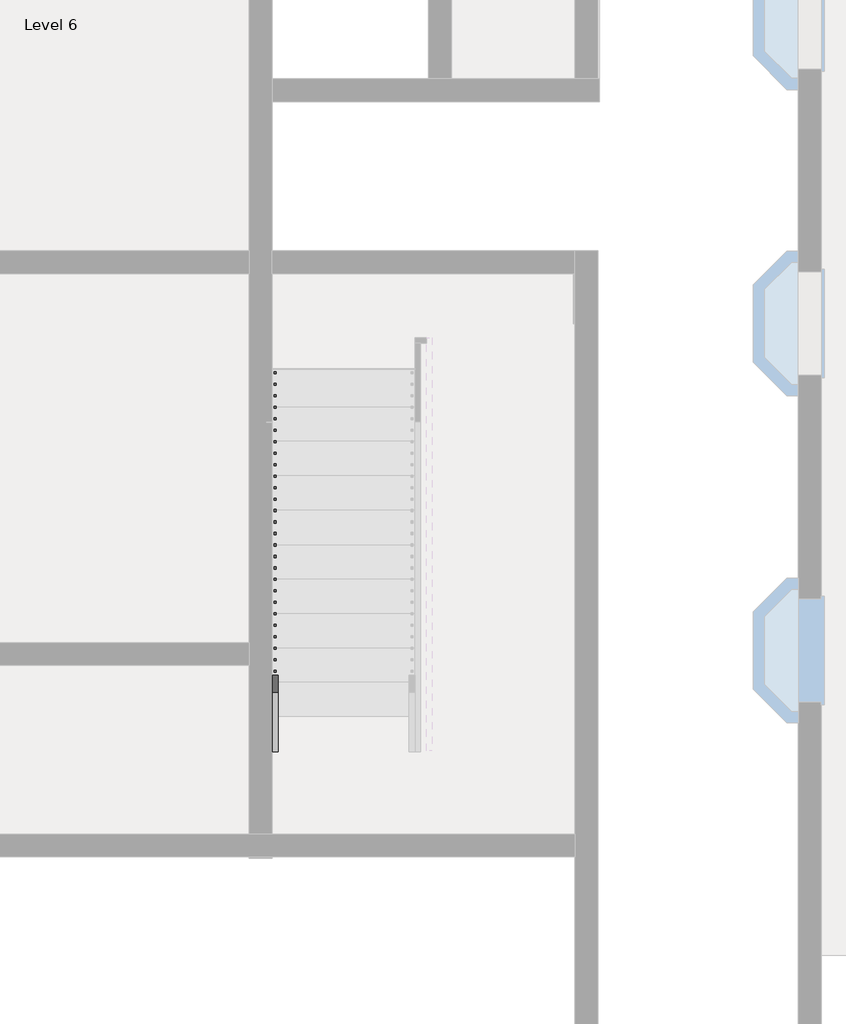
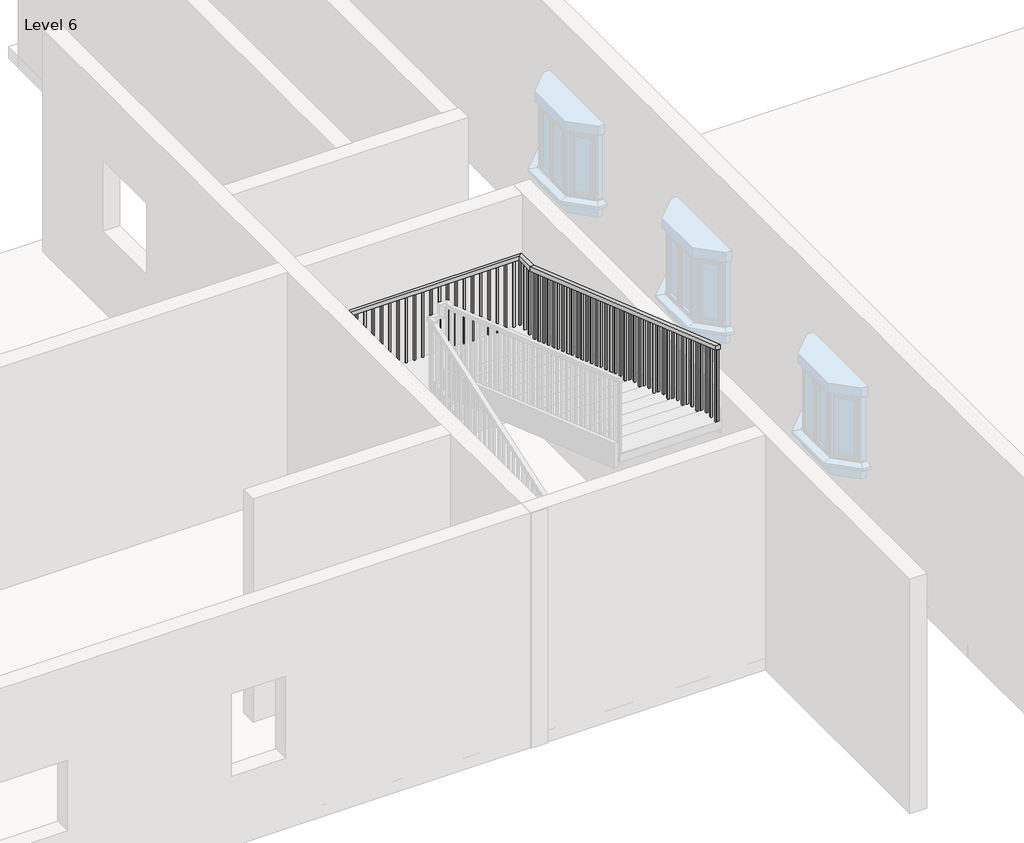
# One storey, part 8 of 14: 1 railing.
"""IFC4 building model written with IfcOpenShell, lengths in millimetres."""

from ifc_helpers import new_model, si_unit, frame, origin, place, context, project, spatial, polyline, outline, extrude, faceted_brep, element, save

model = new_model("IFC4")

# Units and contexts
model_context = context("Model", 3, world=origin())
ifc_project = project(units=[si_unit("LENGTHUNIT", "METRE", prefix="MILLI")], contexts=[model_context])

# Site, building, storey
site = spatial("IfcSite", under=ifc_project)
building = spatial("IfcBuilding", under=site)
storey = spatial("IfcBuildingStorey", under=building, Name="Level 6", Elevation=15240.0)

# Railing
placement = place(None, origin())
element("IfcRailing", 1, ObjectType="Handrail - Rectangular", at=placement, inside=storey, context=model_context, shape_type="SolidModel", body=[
    faceted_brep([(-3857.687215, -9955.5916506, 16259.9076923), (-3857.687215, -9955.5916506, 16206.1602476), (-3806.887215, -9955.5916506, 16206.1602476), (-3806.887215, -9955.5916506, 16259.9076923), (-3857.687215, -6291.6416506, 17526.0), (-3857.687215, -6283.1120276, 17475.2), (-3806.887215, -6283.1120276, 17475.2), (-3806.887215, -6291.6416506, 17526.0), (-3857.687215, -5713.7916506, 17526.0), (-3857.687215, -5713.7916506, 17475.2), (-3806.887215, -5764.5916506, 17475.2), (-3806.887215, -5764.5916506, 17526.0), (-1190.687215, -5713.7916506, 17526.0), (-1190.687215, -5713.7916506, 17475.2), (-1241.487215, -5764.5916506, 17475.2), (-1241.487215, -5764.5916506, 17526.0), (-1190.687215, -5986.8416506, 17526.0), (-1190.687215, -5995.3852679, 17475.2), (-1241.487215, -5995.3852679, 17475.2), (-1241.487215, -5986.8416506, 17526.0), (-1190.687215, -9949.2416506, 18897.6), (-1241.487215, -9949.2416506, 18897.6), (-1241.487215, -9949.2416506, 18843.842594), (-1190.687215, -9949.2416506, 18843.842594)], [[[0, 1, 2, 3]], [[1, 0, 4, 5]], [[2, 1, 5, 6]], [[3, 2, 6, 7]], [[0, 3, 7, 4]], [[5, 4, 8, 9]], [[6, 5, 9, 10]], [[7, 6, 10, 11]], [[4, 7, 11, 8]], [[9, 8, 12, 13]], [[10, 9, 13, 14]], [[11, 10, 14, 15]], [[8, 11, 15, 12]], [[13, 12, 16, 17]], [[14, 13, 17, 18]], [[15, 14, 18, 19]], [[12, 15, 19, 16]], [[20, 21, 22, 23]], [[17, 16, 20, 23]], [[18, 17, 23, 22]], [[19, 18, 22, 21]], [[16, 19, 21, 20]]]),
    extrude(outline(polyline([(-9895.2666506, 18825.1589402), (-9895.2666506, 17877.6923077), (-9914.3166506, 17877.6923077), (-9914.3166506, 18831.7531709), (-9895.2666506, 18825.1589402)])), frame((-1225.612215, 0.0, 0.0), z_axis=(1.0, 0.0, 0.0), x_axis=(0.0, 1.0, 0.0)), (0.0, 0.0, 1.0), 19.05),
    extrude(outline(polyline([(-9793.6666506, 18789.9897094), (-9793.6666506, 17877.6923077), (-9812.7166506, 17877.6923077), (-9812.7166506, 18796.5839402), (-9793.6666506, 18789.9897094)])), frame((-1225.612215, 0.0, 0.0), z_axis=(1.0, 0.0, 0.0), x_axis=(0.0, 1.0, 0.0)), (0.0, 0.0, 1.0), 19.05),
    extrude(outline(polyline([(-9692.0666506, 18754.8204786), (-9692.0666506, 17877.6923077), (-9711.1166506, 17877.6923077), (-9711.1166506, 18761.4147094), (-9692.0666506, 18754.8204786)])), frame((-1225.612215, 0.0, 0.0), z_axis=(1.0, 0.0, 0.0), x_axis=(0.0, 1.0, 0.0)), (0.0, 0.0, 1.0), 19.05),
    extrude(outline(polyline([(-9590.4666506, 18719.6512479), (-9590.4666506, 17772.1846154), (-9609.5166506, 17772.1846154), (-9609.5166506, 18726.2454786), (-9590.4666506, 18719.6512479)])), frame((-1225.612215, 0.0, 0.0), z_axis=(1.0, 0.0, 0.0), x_axis=(0.0, 1.0, 0.0)), (0.0, 0.0, 1.0), 19.05),
    extrude(outline(polyline([(-9488.8666506, 18684.4820171), (-9488.8666506, 17772.1846154), (-9507.9166506, 17772.1846154), (-9507.9166506, 18691.0762479), (-9488.8666506, 18684.4820171)])), frame((-1225.612215, 0.0, 0.0), z_axis=(1.0, 0.0, 0.0), x_axis=(0.0, 1.0, 0.0)), (0.0, 0.0, 1.0), 19.05),
    extrude(outline(polyline([(-9387.2666506, 18649.3127863), (-9387.2666506, 17772.1846154), (-9406.3166506, 17772.1846154), (-9406.3166506, 18655.9070171), (-9387.2666506, 18649.3127863)])), frame((-1225.612215, 0.0, 0.0), z_axis=(1.0, 0.0, 0.0), x_axis=(0.0, 1.0, 0.0)), (0.0, 0.0, 1.0), 19.05),
    extrude(outline(polyline([(-9285.6666506, 18614.1435556), (-9285.6666506, 17666.6769231), (-9304.7166506, 17666.6769231), (-9304.7166506, 18620.7377863), (-9285.6666506, 18614.1435556)])), frame((-1225.612215, 0.0, 0.0), z_axis=(1.0, 0.0, 0.0), x_axis=(0.0, 1.0, 0.0)), (0.0, 0.0, 1.0), 19.05),
    extrude(outline(polyline([(-9184.0666506, 18578.9743248), (-9184.0666506, 17666.6769231), (-9203.1166506, 17666.6769231), (-9203.1166506, 18585.5685556), (-9184.0666506, 18578.9743248)])), frame((-1225.612215, 0.0, 0.0), z_axis=(1.0, 0.0, 0.0), x_axis=(0.0, 1.0, 0.0)), (0.0, 0.0, 1.0), 19.05),
    extrude(outline(polyline([(-9082.4666506, 18543.805094), (-9082.4666506, 17666.6769231), (-9101.5166506, 17666.6769231), (-9101.5166506, 18550.3993248), (-9082.4666506, 18543.805094)])), frame((-1225.612215, 0.0, 0.0), z_axis=(1.0, 0.0, 0.0), x_axis=(0.0, 1.0, 0.0)), (0.0, 0.0, 1.0), 19.05),
    extrude(outline(polyline([(-8980.8666506, 18508.6358632), (-8980.8666506, 17561.1692308), (-8999.9166506, 17561.1692308), (-8999.9166506, 18515.230094), (-8980.8666506, 18508.6358632)])), frame((-1225.612215, 0.0, 0.0), z_axis=(1.0, 0.0, 0.0), x_axis=(0.0, 1.0, 0.0)), (0.0, 0.0, 1.0), 19.05),
    extrude(outline(polyline([(-8879.2666506, 18473.4666325), (-8879.2666506, 17561.1692308), (-8898.3166506, 17561.1692308), (-8898.3166506, 18480.0608632), (-8879.2666506, 18473.4666325)])), frame((-1225.612215, 0.0, 0.0), z_axis=(1.0, 0.0, 0.0), x_axis=(0.0, 1.0, 0.0)), (0.0, 0.0, 1.0), 19.05),
    extrude(outline(polyline([(-8777.6666506, 18438.2974017), (-8777.6666506, 17561.1692308), (-8796.7166506, 17561.1692308), (-8796.7166506, 18444.8916325), (-8777.6666506, 18438.2974017)])), frame((-1225.612215, 0.0, 0.0), z_axis=(1.0, 0.0, 0.0), x_axis=(0.0, 1.0, 0.0)), (0.0, 0.0, 1.0), 19.05),
    extrude(outline(polyline([(-8676.0666506, 18403.1281709), (-8676.0666506, 17455.6615385), (-8695.1166506, 17455.6615385), (-8695.1166506, 18409.7224017), (-8676.0666506, 18403.1281709)])), frame((-1225.612215, 0.0, 0.0), z_axis=(1.0, 0.0, 0.0), x_axis=(0.0, 1.0, 0.0)), (0.0, 0.0, 1.0), 19.05),
    extrude(outline(polyline([(-8574.4666506, 18367.9589402), (-8574.4666506, 17455.6615385), (-8593.5166506, 17455.6615385), (-8593.5166506, 18374.5531709), (-8574.4666506, 18367.9589402)])), frame((-1225.612215, 0.0, 0.0), z_axis=(1.0, 0.0, 0.0), x_axis=(0.0, 1.0, 0.0)), (0.0, 0.0, 1.0), 19.05),
    extrude(outline(polyline([(-8472.8666506, 18332.7897094), (-8472.8666506, 17455.6615385), (-8491.9166506, 17455.6615385), (-8491.9166506, 18339.3839402), (-8472.8666506, 18332.7897094)])), frame((-1225.612215, 0.0, 0.0), z_axis=(1.0, 0.0, 0.0), x_axis=(0.0, 1.0, 0.0)), (0.0, 0.0, 1.0), 19.05),
    extrude(outline(polyline([(-8371.2666506, 18297.6204786), (-8371.2666506, 17350.1538462), (-8390.3166506, 17350.1538462), (-8390.3166506, 18304.2147094), (-8371.2666506, 18297.6204786)])), frame((-1225.612215, 0.0, 0.0), z_axis=(1.0, 0.0, 0.0), x_axis=(0.0, 1.0, 0.0)), (0.0, 0.0, 1.0), 19.05),
    extrude(outline(polyline([(-8269.6666506, 18262.4512479), (-8269.6666506, 17350.1538462), (-8288.7166506, 17350.1538462), (-8288.7166506, 18269.0454786), (-8269.6666506, 18262.4512479)])), frame((-1225.612215, 0.0, 0.0), z_axis=(1.0, 0.0, 0.0), x_axis=(0.0, 1.0, 0.0)), (0.0, 0.0, 1.0), 19.05),
    extrude(outline(polyline([(-8168.0666506, 18227.2820171), (-8168.0666506, 17350.1538462), (-8187.1166506, 17350.1538462), (-8187.1166506, 18233.8762479), (-8168.0666506, 18227.2820171)])), frame((-1225.612215, 0.0, 0.0), z_axis=(1.0, 0.0, 0.0), x_axis=(0.0, 1.0, 0.0)), (0.0, 0.0, 1.0), 19.05),
    extrude(outline(polyline([(-8066.4666506, 18192.1127863), (-8066.4666506, 17244.6461538), (-8085.5166506, 17244.6461538), (-8085.5166506, 18198.7070171), (-8066.4666506, 18192.1127863)])), frame((-1225.612215, 0.0, 0.0), z_axis=(1.0, 0.0, 0.0), x_axis=(0.0, 1.0, 0.0)), (0.0, 0.0, 1.0), 19.05),
    extrude(outline(polyline([(-7964.8666506, 18156.9435556), (-7964.8666506, 17244.6461538), (-7983.9166506, 17244.6461538), (-7983.9166506, 18163.5377863), (-7964.8666506, 18156.9435556)])), frame((-1225.612215, 0.0, 0.0), z_axis=(1.0, 0.0, 0.0), x_axis=(0.0, 1.0, 0.0)), (0.0, 0.0, 1.0), 19.05),
    extrude(outline(polyline([(-7863.2666506, 18121.7743248), (-7863.2666506, 17244.6461538), (-7882.3166506, 17244.6461538), (-7882.3166506, 18128.3685556), (-7863.2666506, 18121.7743248)])), frame((-1225.612215, 0.0, 0.0), z_axis=(1.0, 0.0, 0.0), x_axis=(0.0, 1.0, 0.0)), (0.0, 0.0, 1.0), 19.05),
    extrude(outline(polyline([(-7761.6666506, 18086.605094), (-7761.6666506, 17139.1384615), (-7780.7166506, 17139.1384615), (-7780.7166506, 18093.1993248), (-7761.6666506, 18086.605094)])), frame((-1225.612215, 0.0, 0.0), z_axis=(1.0, 0.0, 0.0), x_axis=(0.0, 1.0, 0.0)), (0.0, 0.0, 1.0), 19.05),
    extrude(outline(polyline([(-7660.0666506, 18051.4358632), (-7660.0666506, 17139.1384615), (-7679.1166506, 17139.1384615), (-7679.1166506, 18058.030094), (-7660.0666506, 18051.4358632)])), frame((-1225.612215, 0.0, 0.0), z_axis=(1.0, 0.0, 0.0), x_axis=(0.0, 1.0, 0.0)), (0.0, 0.0, 1.0), 19.05),
    extrude(outline(polyline([(-7558.4666506, 18016.2666325), (-7558.4666506, 17139.1384615), (-7577.5166506, 17139.1384615), (-7577.5166506, 18022.8608632), (-7558.4666506, 18016.2666325)])), frame((-1225.612215, 0.0, 0.0), z_axis=(1.0, 0.0, 0.0), x_axis=(0.0, 1.0, 0.0)), (0.0, 0.0, 1.0), 19.05),
    extrude(outline(polyline([(-7456.8666506, 17981.0974017), (-7456.8666506, 17033.6307692), (-7475.9166506, 17033.6307692), (-7475.9166506, 17987.6916325), (-7456.8666506, 17981.0974017)])), frame((-1225.612215, 0.0, 0.0), z_axis=(1.0, 0.0, 0.0), x_axis=(0.0, 1.0, 0.0)), (0.0, 0.0, 1.0), 19.05),
    extrude(outline(polyline([(-7355.2666506, 17945.9281709), (-7355.2666506, 17033.6307692), (-7374.3166506, 17033.6307692), (-7374.3166506, 17952.5224017), (-7355.2666506, 17945.9281709)])), frame((-1225.612215, 0.0, 0.0), z_axis=(1.0, 0.0, 0.0), x_axis=(0.0, 1.0, 0.0)), (0.0, 0.0, 1.0), 19.05),
    extrude(outline(polyline([(-7253.6666506, 17910.7589402), (-7253.6666506, 17033.6307692), (-7272.7166506, 17033.6307692), (-7272.7166506, 17917.3531709), (-7253.6666506, 17910.7589402)])), frame((-1225.612215, 0.0, 0.0), z_axis=(1.0, 0.0, 0.0), x_axis=(0.0, 1.0, 0.0)), (0.0, 0.0, 1.0), 19.05),
    extrude(outline(polyline([(-7152.0666506, 17875.5897094), (-7152.0666506, 16928.1230769), (-7171.1166506, 16928.1230769), (-7171.1166506, 17882.1839402), (-7152.0666506, 17875.5897094)])), frame((-1225.612215, 0.0, 0.0), z_axis=(1.0, 0.0, 0.0), x_axis=(0.0, 1.0, 0.0)), (0.0, 0.0, 1.0), 19.05),
    extrude(outline(polyline([(-7050.4666506, 17840.4204786), (-7050.4666506, 16928.1230769), (-7069.5166506, 16928.1230769), (-7069.5166506, 17847.0147094), (-7050.4666506, 17840.4204786)])), frame((-1225.612215, 0.0, 0.0), z_axis=(1.0, 0.0, 0.0), x_axis=(0.0, 1.0, 0.0)), (0.0, 0.0, 1.0), 19.05),
    extrude(outline(polyline([(-6948.8666506, 17805.2512479), (-6948.8666506, 16928.1230769), (-6967.9166506, 16928.1230769), (-6967.9166506, 17811.8454786), (-6948.8666506, 17805.2512479)])), frame((-1225.612215, 0.0, 0.0), z_axis=(1.0, 0.0, 0.0), x_axis=(0.0, 1.0, 0.0)), (0.0, 0.0, 1.0), 19.05),
    extrude(outline(polyline([(-6847.2666506, 17770.0820171), (-6847.2666506, 16822.6153846), (-6866.3166506, 16822.6153846), (-6866.3166506, 17776.6762479), (-6847.2666506, 17770.0820171)])), frame((-1225.612215, 0.0, 0.0), z_axis=(1.0, 0.0, 0.0), x_axis=(0.0, 1.0, 0.0)), (0.0, 0.0, 1.0), 19.05),
    extrude(outline(polyline([(-6745.6666506, 17734.9127863), (-6745.6666506, 16822.6153846), (-6764.7166506, 16822.6153846), (-6764.7166506, 17741.5070171), (-6745.6666506, 17734.9127863)])), frame((-1225.612215, 0.0, 0.0), z_axis=(1.0, 0.0, 0.0), x_axis=(0.0, 1.0, 0.0)), (0.0, 0.0, 1.0), 19.05),
    extrude(outline(polyline([(-6644.0666506, 17699.7435556), (-6644.0666506, 16822.6153846), (-6663.1166506, 16822.6153846), (-6663.1166506, 17706.3377863), (-6644.0666506, 17699.7435556)])), frame((-1225.612215, 0.0, 0.0), z_axis=(1.0, 0.0, 0.0), x_axis=(0.0, 1.0, 0.0)), (0.0, 0.0, 1.0), 19.05),
    extrude(outline(polyline([(-6542.4666506, 17664.5743248), (-6542.4666506, 16717.1076923), (-6561.5166506, 16717.1076923), (-6561.5166506, 17671.1685556), (-6542.4666506, 17664.5743248)])), frame((-1225.612215, 0.0, 0.0), z_axis=(1.0, 0.0, 0.0), x_axis=(0.0, 1.0, 0.0)), (0.0, 0.0, 1.0), 19.05),
    extrude(outline(polyline([(-6440.8666506, 17629.405094), (-6440.8666506, 16717.1076923), (-6459.9166506, 16717.1076923), (-6459.9166506, 17635.9993248), (-6440.8666506, 17629.405094)])), frame((-1225.612215, 0.0, 0.0), z_axis=(1.0, 0.0, 0.0), x_axis=(0.0, 1.0, 0.0)), (0.0, 0.0, 1.0), 19.05),
    extrude(outline(polyline([(-6339.2666506, 17594.2358632), (-6339.2666506, 16717.1076923), (-6358.3166506, 16717.1076923), (-6358.3166506, 17600.830094), (-6339.2666506, 17594.2358632)])), frame((-1225.612215, 0.0, 0.0), z_axis=(1.0, 0.0, 0.0), x_axis=(0.0, 1.0, 0.0)), (0.0, 0.0, 1.0), 19.05),
    extrude(outline(polyline([(-6237.6666506, 17559.0666325), (-6237.6666506, 16611.6), (-6256.7166506, 16611.6), (-6256.7166506, 17565.6608632), (-6237.6666506, 17559.0666325)])), frame((-1225.612215, 0.0, 0.0), z_axis=(1.0, 0.0, 0.0), x_axis=(0.0, 1.0, 0.0)), (0.0, 0.0, 1.0), 19.05),
    extrude(outline(polyline([(-6136.0666506, 17523.8974017), (-6136.0666506, 16611.6), (-6155.1166506, 16611.6), (-6155.1166506, 17530.4916325), (-6136.0666506, 17523.8974017)])), frame((-1225.612215, 0.0, 0.0), z_axis=(1.0, 0.0, 0.0), x_axis=(0.0, 1.0, 0.0)), (0.0, 0.0, 1.0), 19.05),
    extrude(outline(polyline([(-6034.4666506, 17488.7281709), (-6034.4666506, 16611.6), (-6053.5166506, 16611.6), (-6053.5166506, 17495.3224017), (-6034.4666506, 17488.7281709)])), frame((-1225.612215, 0.0, 0.0), z_axis=(1.0, 0.0, 0.0), x_axis=(0.0, 1.0, 0.0)), (0.0, 0.0, 1.0), 19.05),
    extrude(outline(polyline([(-1206.562215, -5932.8666506), (-1206.562215, -5951.9166506), (-1225.612215, -5951.9166506), (-1225.612215, -5932.8666506), (-1206.562215, -5932.8666506)])), frame((0.0, 0.0, 16611.6), z_axis=(0.0, 0.0, 1.0), x_axis=(1.0, 0.0, 0.0)), (0.0, 0.0, 1.0), 863.6),
    extrude(outline(polyline([(-1206.562215, -5831.2666506), (-1206.562215, -5850.3166506), (-1225.612215, -5850.3166506), (-1225.612215, -5831.2666506), (-1206.562215, -5831.2666506)])), frame((0.0, 0.0, 16611.6), z_axis=(0.0, 0.0, 1.0), x_axis=(1.0, 0.0, 0.0)), (0.0, 0.0, 1.0), 863.6),
    extrude(outline(polyline([(-1301.812215, -5729.6666506), (-1282.762215, -5729.6666506), (-1282.762215, -5748.7166506), (-1301.812215, -5748.7166506), (-1301.812215, -5729.6666506)])), frame((0.0, 0.0, 16611.6), z_axis=(0.0, 0.0, 1.0), x_axis=(1.0, 0.0, 0.0)), (0.0, 0.0, 1.0), 863.6),
    extrude(outline(polyline([(-1403.412215, -5729.6666506), (-1384.362215, -5729.6666506), (-1384.362215, -5748.7166506), (-1403.412215, -5748.7166506), (-1403.412215, -5729.6666506)])), frame((0.0, 0.0, 16611.6), z_axis=(0.0, 0.0, 1.0), x_axis=(1.0, 0.0, 0.0)), (0.0, 0.0, 1.0), 863.6),
    extrude(outline(polyline([(-1505.012215, -5729.6666506), (-1485.962215, -5729.6666506), (-1485.962215, -5748.7166506), (-1505.012215, -5748.7166506), (-1505.012215, -5729.6666506)])), frame((0.0, 0.0, 16611.6), z_axis=(0.0, 0.0, 1.0), x_axis=(1.0, 0.0, 0.0)), (0.0, 0.0, 1.0), 863.6),
    extrude(outline(polyline([(-1606.612215, -5729.6666506), (-1587.562215, -5729.6666506), (-1587.562215, -5748.7166506), (-1606.612215, -5748.7166506), (-1606.612215, -5729.6666506)])), frame((0.0, 0.0, 16611.6), z_axis=(0.0, 0.0, 1.0), x_axis=(1.0, 0.0, 0.0)), (0.0, 0.0, 1.0), 863.6),
    extrude(outline(polyline([(-1708.212215, -5729.6666506), (-1689.162215, -5729.6666506), (-1689.162215, -5748.7166506), (-1708.212215, -5748.7166506), (-1708.212215, -5729.6666506)])), frame((0.0, 0.0, 16611.6), z_axis=(0.0, 0.0, 1.0), x_axis=(1.0, 0.0, 0.0)), (0.0, 0.0, 1.0), 863.6),
    extrude(outline(polyline([(-1809.812215, -5729.6666506), (-1790.762215, -5729.6666506), (-1790.762215, -5748.7166506), (-1809.812215, -5748.7166506), (-1809.812215, -5729.6666506)])), frame((0.0, 0.0, 16611.6), z_axis=(0.0, 0.0, 1.0), x_axis=(1.0, 0.0, 0.0)), (0.0, 0.0, 1.0), 863.6),
    extrude(outline(polyline([(-1911.412215, -5729.6666506), (-1892.362215, -5729.6666506), (-1892.362215, -5748.7166506), (-1911.412215, -5748.7166506), (-1911.412215, -5729.6666506)])), frame((0.0, 0.0, 16611.6), z_axis=(0.0, 0.0, 1.0), x_axis=(1.0, 0.0, 0.0)), (0.0, 0.0, 1.0), 863.6),
    extrude(outline(polyline([(-2013.012215, -5729.6666506), (-1993.962215, -5729.6666506), (-1993.962215, -5748.7166506), (-2013.012215, -5748.7166506), (-2013.012215, -5729.6666506)])), frame((0.0, 0.0, 16611.6), z_axis=(0.0, 0.0, 1.0), x_axis=(1.0, 0.0, 0.0)), (0.0, 0.0, 1.0), 863.6),
    extrude(outline(polyline([(-2114.612215, -5729.6666506), (-2095.562215, -5729.6666506), (-2095.562215, -5748.7166506), (-2114.612215, -5748.7166506), (-2114.612215, -5729.6666506)])), frame((0.0, 0.0, 16611.6), z_axis=(0.0, 0.0, 1.0), x_axis=(1.0, 0.0, 0.0)), (0.0, 0.0, 1.0), 863.6),
    extrude(outline(polyline([(-2216.212215, -5729.6666506), (-2197.162215, -5729.6666506), (-2197.162215, -5748.7166506), (-2216.212215, -5748.7166506), (-2216.212215, -5729.6666506)])), frame((0.0, 0.0, 16611.6), z_axis=(0.0, 0.0, 1.0), x_axis=(1.0, 0.0, 0.0)), (0.0, 0.0, 1.0), 863.6),
    extrude(outline(polyline([(-2317.812215, -5729.6666506), (-2298.762215, -5729.6666506), (-2298.762215, -5748.7166506), (-2317.812215, -5748.7166506), (-2317.812215, -5729.6666506)])), frame((0.0, 0.0, 16611.6), z_axis=(0.0, 0.0, 1.0), x_axis=(1.0, 0.0, 0.0)), (0.0, 0.0, 1.0), 863.6),
    extrude(outline(polyline([(-2419.412215, -5729.6666506), (-2400.362215, -5729.6666506), (-2400.362215, -5748.7166506), (-2419.412215, -5748.7166506), (-2419.412215, -5729.6666506)])), frame((0.0, 0.0, 16611.6), z_axis=(0.0, 0.0, 1.0), x_axis=(1.0, 0.0, 0.0)), (0.0, 0.0, 1.0), 863.6),
    extrude(outline(polyline([(-2521.012215, -5729.6666506), (-2501.962215, -5729.6666506), (-2501.962215, -5748.7166506), (-2521.012215, -5748.7166506), (-2521.012215, -5729.6666506)])), frame((0.0, 0.0, 16611.6), z_axis=(0.0, 0.0, 1.0), x_axis=(1.0, 0.0, 0.0)), (0.0, 0.0, 1.0), 863.6),
    extrude(outline(polyline([(-2622.612215, -5729.6666506), (-2603.562215, -5729.6666506), (-2603.562215, -5748.7166506), (-2622.612215, -5748.7166506), (-2622.612215, -5729.6666506)])), frame((0.0, 0.0, 16611.6), z_axis=(0.0, 0.0, 1.0), x_axis=(1.0, 0.0, 0.0)), (0.0, 0.0, 1.0), 863.6),
    extrude(outline(polyline([(-2724.212215, -5729.6666506), (-2705.162215, -5729.6666506), (-2705.162215, -5748.7166506), (-2724.212215, -5748.7166506), (-2724.212215, -5729.6666506)])), frame((0.0, 0.0, 16611.6), z_axis=(0.0, 0.0, 1.0), x_axis=(1.0, 0.0, 0.0)), (0.0, 0.0, 1.0), 863.6),
    extrude(outline(polyline([(-2825.812215, -5729.6666506), (-2806.762215, -5729.6666506), (-2806.762215, -5748.7166506), (-2825.812215, -5748.7166506), (-2825.812215, -5729.6666506)])), frame((0.0, 0.0, 16611.6), z_axis=(0.0, 0.0, 1.0), x_axis=(1.0, 0.0, 0.0)), (0.0, 0.0, 1.0), 863.6),
    extrude(outline(polyline([(-2927.412215, -5729.6666506), (-2908.362215, -5729.6666506), (-2908.362215, -5748.7166506), (-2927.412215, -5748.7166506), (-2927.412215, -5729.6666506)])), frame((0.0, 0.0, 16611.6), z_axis=(0.0, 0.0, 1.0), x_axis=(1.0, 0.0, 0.0)), (0.0, 0.0, 1.0), 863.6),
    extrude(outline(polyline([(-3029.012215, -5729.6666506), (-3009.962215, -5729.6666506), (-3009.962215, -5748.7166506), (-3029.012215, -5748.7166506), (-3029.012215, -5729.6666506)])), frame((0.0, 0.0, 16611.6), z_axis=(0.0, 0.0, 1.0), x_axis=(1.0, 0.0, 0.0)), (0.0, 0.0, 1.0), 863.6),
    extrude(outline(polyline([(-3130.612215, -5729.6666506), (-3111.562215, -5729.6666506), (-3111.562215, -5748.7166506), (-3130.612215, -5748.7166506), (-3130.612215, -5729.6666506)])), frame((0.0, 0.0, 16611.6), z_axis=(0.0, 0.0, 1.0), x_axis=(1.0, 0.0, 0.0)), (0.0, 0.0, 1.0), 863.6),
    extrude(outline(polyline([(-3232.212215, -5729.6666506), (-3213.162215, -5729.6666506), (-3213.162215, -5748.7166506), (-3232.212215, -5748.7166506), (-3232.212215, -5729.6666506)])), frame((0.0, 0.0, 16611.6), z_axis=(0.0, 0.0, 1.0), x_axis=(1.0, 0.0, 0.0)), (0.0, 0.0, 1.0), 863.6),
    extrude(outline(polyline([(-3333.812215, -5729.6666506), (-3314.762215, -5729.6666506), (-3314.762215, -5748.7166506), (-3333.812215, -5748.7166506), (-3333.812215, -5729.6666506)])), frame((0.0, 0.0, 16611.6), z_axis=(0.0, 0.0, 1.0), x_axis=(1.0, 0.0, 0.0)), (0.0, 0.0, 1.0), 863.6),
    extrude(outline(polyline([(-3435.412215, -5729.6666506), (-3416.362215, -5729.6666506), (-3416.362215, -5748.7166506), (-3435.412215, -5748.7166506), (-3435.412215, -5729.6666506)])), frame((0.0, 0.0, 16611.6), z_axis=(0.0, 0.0, 1.0), x_axis=(1.0, 0.0, 0.0)), (0.0, 0.0, 1.0), 863.6),
    extrude(outline(polyline([(-3537.012215, -5729.6666506), (-3517.962215, -5729.6666506), (-3517.962215, -5748.7166506), (-3537.012215, -5748.7166506), (-3537.012215, -5729.6666506)])), frame((0.0, 0.0, 16611.6), z_axis=(0.0, 0.0, 1.0), x_axis=(1.0, 0.0, 0.0)), (0.0, 0.0, 1.0), 863.6),
    extrude(outline(polyline([(-3638.612215, -5729.6666506), (-3619.562215, -5729.6666506), (-3619.562215, -5748.7166506), (-3638.612215, -5748.7166506), (-3638.612215, -5729.6666506)])), frame((0.0, 0.0, 16611.6), z_axis=(0.0, 0.0, 1.0), x_axis=(1.0, 0.0, 0.0)), (0.0, 0.0, 1.0), 863.6),
    extrude(outline(polyline([(-3740.212215, -5729.6666506), (-3721.162215, -5729.6666506), (-3721.162215, -5748.7166506), (-3740.212215, -5748.7166506), (-3740.212215, -5729.6666506)])), frame((0.0, 0.0, 16611.6), z_axis=(0.0, 0.0, 1.0), x_axis=(1.0, 0.0, 0.0)), (0.0, 0.0, 1.0), 863.6),
    extrude(outline(polyline([(-3841.812215, -5799.5166506), (-3841.812215, -5780.4666506), (-3822.762215, -5780.4666506), (-3822.762215, -5799.5166506), (-3841.812215, -5799.5166506)])), frame((0.0, 0.0, 16611.6), z_axis=(0.0, 0.0, 1.0), x_axis=(1.0, 0.0, 0.0)), (0.0, 0.0, 1.0), 863.6),
    extrude(outline(polyline([(-3841.812215, -5901.1166506), (-3841.812215, -5882.0666506), (-3822.762215, -5882.0666506), (-3822.762215, -5901.1166506), (-3841.812215, -5901.1166506)])), frame((0.0, 0.0, 16611.6), z_axis=(0.0, 0.0, 1.0), x_axis=(1.0, 0.0, 0.0)), (0.0, 0.0, 1.0), 863.6),
    extrude(outline(polyline([(-3841.812215, -6002.7166506), (-3841.812215, -5983.6666506), (-3822.762215, -5983.6666506), (-3822.762215, -6002.7166506), (-3841.812215, -6002.7166506)])), frame((0.0, 0.0, 16611.6), z_axis=(0.0, 0.0, 1.0), x_axis=(1.0, 0.0, 0.0)), (0.0, 0.0, 1.0), 863.6),
    extrude(outline(polyline([(-3841.812215, -6104.3166506), (-3841.812215, -6085.2666506), (-3822.762215, -6085.2666506), (-3822.762215, -6104.3166506), (-3841.812215, -6104.3166506)])), frame((0.0, 0.0, 16611.6), z_axis=(0.0, 0.0, 1.0), x_axis=(1.0, 0.0, 0.0)), (0.0, 0.0, 1.0), 863.6),
    extrude(outline(polyline([(-3841.812215, -6205.9166506), (-3841.812215, -6186.8666506), (-3822.762215, -6186.8666506), (-3822.762215, -6205.9166506), (-3841.812215, -6205.9166506)])), frame((0.0, 0.0, 16611.6), z_axis=(0.0, 0.0, 1.0), x_axis=(1.0, 0.0, 0.0)), (0.0, 0.0, 1.0), 863.6),
    extrude(outline(polyline([(-6288.4666506, 17473.349689), (-6288.4666506, 16506.0923077), (-6307.5166506, 16506.0923077), (-6307.5166506, 17466.7668867), (-6288.4666506, 17473.349689)])), frame((-3841.812215, 0.0, 0.0), z_axis=(1.0, 0.0, 0.0), x_axis=(0.0, 1.0, 0.0)), (0.0, 0.0, 1.0), 19.05),
    extrude(outline(polyline([(-6390.0666506, 17438.2414101), (-6390.0666506, 16506.0923077), (-6409.1166506, 16506.0923077), (-6409.1166506, 17431.6586078), (-6390.0666506, 17438.2414101)])), frame((-3841.812215, 0.0, 0.0), z_axis=(1.0, 0.0, 0.0), x_axis=(0.0, 1.0, 0.0)), (0.0, 0.0, 1.0), 19.05),
    extrude(outline(polyline([(-6491.6666506, 17403.1331312), (-6491.6666506, 16506.0923077), (-6510.7166506, 16506.0923077), (-6510.7166506, 17396.5503289), (-6491.6666506, 17403.1331312)])), frame((-3841.812215, 0.0, 0.0), z_axis=(1.0, 0.0, 0.0), x_axis=(0.0, 1.0, 0.0)), (0.0, 0.0, 1.0), 19.05),
    extrude(outline(polyline([(-6593.2666506, 17368.0248523), (-6593.2666506, 16400.5846154), (-6612.3166506, 16400.5846154), (-6612.3166506, 17361.44205), (-6593.2666506, 17368.0248523)])), frame((-3841.812215, 0.0, 0.0), z_axis=(1.0, 0.0, 0.0), x_axis=(0.0, 1.0, 0.0)), (0.0, 0.0, 1.0), 19.05),
    extrude(outline(polyline([(-6694.8666506, 17332.9165734), (-6694.8666506, 16400.5846154), (-6713.9166506, 16400.5846154), (-6713.9166506, 17326.3337711), (-6694.8666506, 17332.9165734)])), frame((-3841.812215, 0.0, 0.0), z_axis=(1.0, 0.0, 0.0), x_axis=(0.0, 1.0, 0.0)), (0.0, 0.0, 1.0), 19.05),
    extrude(outline(polyline([(-6796.4666506, 17297.8082945), (-6796.4666506, 16400.5846154), (-6815.5166506, 16400.5846154), (-6815.5166506, 17291.2254922), (-6796.4666506, 17297.8082945)])), frame((-3841.812215, 0.0, 0.0), z_axis=(1.0, 0.0, 0.0), x_axis=(0.0, 1.0, 0.0)), (0.0, 0.0, 1.0), 19.05),
    extrude(outline(polyline([(-6898.0666506, 17262.7000156), (-6898.0666506, 16295.0769231), (-6917.1166506, 16295.0769231), (-6917.1166506, 17256.1172133), (-6898.0666506, 17262.7000156)])), frame((-3841.812215, 0.0, 0.0), z_axis=(1.0, 0.0, 0.0), x_axis=(0.0, 1.0, 0.0)), (0.0, 0.0, 1.0), 19.05),
    extrude(outline(polyline([(-6999.6666506, 17227.5917367), (-6999.6666506, 16295.0769231), (-7018.7166506, 16295.0769231), (-7018.7166506, 17221.0089344), (-6999.6666506, 17227.5917367)])), frame((-3841.812215, 0.0, 0.0), z_axis=(1.0, 0.0, 0.0), x_axis=(0.0, 1.0, 0.0)), (0.0, 0.0, 1.0), 19.05),
    extrude(outline(polyline([(-7101.2666506, 17192.4834578), (-7101.2666506, 16295.0769231), (-7120.3166506, 16295.0769231), (-7120.3166506, 17185.9006556), (-7101.2666506, 17192.4834578)])), frame((-3841.812215, 0.0, 0.0), z_axis=(1.0, 0.0, 0.0), x_axis=(0.0, 1.0, 0.0)), (0.0, 0.0, 1.0), 19.05),
    extrude(outline(polyline([(-7202.8666506, 17157.3751789), (-7202.8666506, 16189.5692308), (-7221.9166506, 16189.5692308), (-7221.9166506, 17150.7923767), (-7202.8666506, 17157.3751789)])), frame((-3841.812215, 0.0, 0.0), z_axis=(1.0, 0.0, 0.0), x_axis=(0.0, 1.0, 0.0)), (0.0, 0.0, 1.0), 19.05),
    extrude(outline(polyline([(-7304.4666506, 17122.2669001), (-7304.4666506, 16189.5692308), (-7323.5166506, 16189.5692308), (-7323.5166506, 17115.6840978), (-7304.4666506, 17122.2669001)])), frame((-3841.812215, 0.0, 0.0), z_axis=(1.0, 0.0, 0.0), x_axis=(0.0, 1.0, 0.0)), (0.0, 0.0, 1.0), 19.05),
    extrude(outline(polyline([(-7406.0666506, 17087.1586212), (-7406.0666506, 16189.5692308), (-7425.1166506, 16189.5692308), (-7425.1166506, 17080.5758189), (-7406.0666506, 17087.1586212)])), frame((-3841.812215, 0.0, 0.0), z_axis=(1.0, 0.0, 0.0), x_axis=(0.0, 1.0, 0.0)), (0.0, 0.0, 1.0), 19.05),
    extrude(outline(polyline([(-7507.6666506, 17052.0503423), (-7507.6666506, 16084.0615385), (-7526.7166506, 16084.0615385), (-7526.7166506, 17045.46754), (-7507.6666506, 17052.0503423)])), frame((-3841.812215, 0.0, 0.0), z_axis=(1.0, 0.0, 0.0), x_axis=(0.0, 1.0, 0.0)), (0.0, 0.0, 1.0), 19.05),
    extrude(outline(polyline([(-7609.2666506, 17016.9420634), (-7609.2666506, 16084.0615385), (-7628.3166506, 16084.0615385), (-7628.3166506, 17010.3592611), (-7609.2666506, 17016.9420634)])), frame((-3841.812215, 0.0, 0.0), z_axis=(1.0, 0.0, 0.0), x_axis=(0.0, 1.0, 0.0)), (0.0, 0.0, 1.0), 19.05),
    extrude(outline(polyline([(-7710.8666506, 16981.8337845), (-7710.8666506, 16084.0615385), (-7729.9166506, 16084.0615385), (-7729.9166506, 16975.2509822), (-7710.8666506, 16981.8337845)])), frame((-3841.812215, 0.0, 0.0), z_axis=(1.0, 0.0, 0.0), x_axis=(0.0, 1.0, 0.0)), (0.0, 0.0, 1.0), 19.05),
    extrude(outline(polyline([(-7812.4666506, 16946.7255056), (-7812.4666506, 15978.5538462), (-7831.5166506, 15978.5538462), (-7831.5166506, 16940.1427033), (-7812.4666506, 16946.7255056)])), frame((-3841.812215, 0.0, 0.0), z_axis=(1.0, 0.0, 0.0), x_axis=(0.0, 1.0, 0.0)), (0.0, 0.0, 1.0), 19.05),
    extrude(outline(polyline([(-7914.0666506, 16911.6172267), (-7914.0666506, 15978.5538462), (-7933.1166506, 15978.5538462), (-7933.1166506, 16905.0344244), (-7914.0666506, 16911.6172267)])), frame((-3841.812215, 0.0, 0.0), z_axis=(1.0, 0.0, 0.0), x_axis=(0.0, 1.0, 0.0)), (0.0, 0.0, 1.0), 19.05),
    extrude(outline(polyline([(-8015.6666506, 16876.5089478), (-8015.6666506, 15978.5538462), (-8034.7166506, 15978.5538462), (-8034.7166506, 16869.9261455), (-8015.6666506, 16876.5089478)])), frame((-3841.812215, 0.0, 0.0), z_axis=(1.0, 0.0, 0.0), x_axis=(0.0, 1.0, 0.0)), (0.0, 0.0, 1.0), 19.05),
    extrude(outline(polyline([(-8117.2666506, 16841.4006689), (-8117.2666506, 15873.0461538), (-8136.3166506, 15873.0461538), (-8136.3166506, 16834.8178666), (-8117.2666506, 16841.4006689)])), frame((-3841.812215, 0.0, 0.0), z_axis=(1.0, 0.0, 0.0), x_axis=(0.0, 1.0, 0.0)), (0.0, 0.0, 1.0), 19.05),
    extrude(outline(polyline([(-8218.8666506, 16806.29239), (-8218.8666506, 15873.0461538), (-8237.9166506, 15873.0461538), (-8237.9166506, 16799.7095877), (-8218.8666506, 16806.29239)])), frame((-3841.812215, 0.0, 0.0), z_axis=(1.0, 0.0, 0.0), x_axis=(0.0, 1.0, 0.0)), (0.0, 0.0, 1.0), 19.05),
    extrude(outline(polyline([(-8320.4666506, 16771.1841111), (-8320.4666506, 15873.0461538), (-8339.5166506, 15873.0461538), (-8339.5166506, 16764.6013088), (-8320.4666506, 16771.1841111)])), frame((-3841.812215, 0.0, 0.0), z_axis=(1.0, 0.0, 0.0), x_axis=(0.0, 1.0, 0.0)), (0.0, 0.0, 1.0), 19.05),
    extrude(outline(polyline([(-8422.0666506, 16736.0758322), (-8422.0666506, 15767.5384615), (-8441.1166506, 15767.5384615), (-8441.1166506, 16729.4930299), (-8422.0666506, 16736.0758322)])), frame((-3841.812215, 0.0, 0.0), z_axis=(1.0, 0.0, 0.0), x_axis=(0.0, 1.0, 0.0)), (0.0, 0.0, 1.0), 19.05),
    extrude(outline(polyline([(-8523.6666506, 16700.9675533), (-8523.6666506, 15767.5384615), (-8542.7166506, 15767.5384615), (-8542.7166506, 16694.384751), (-8523.6666506, 16700.9675533)])), frame((-3841.812215, 0.0, 0.0), z_axis=(1.0, 0.0, 0.0), x_axis=(0.0, 1.0, 0.0)), (0.0, 0.0, 1.0), 19.05),
    extrude(outline(polyline([(-8625.2666506, 16665.8592744), (-8625.2666506, 15767.5384615), (-8644.3166506, 15767.5384615), (-8644.3166506, 16659.2764721), (-8625.2666506, 16665.8592744)])), frame((-3841.812215, 0.0, 0.0), z_axis=(1.0, 0.0, 0.0), x_axis=(0.0, 1.0, 0.0)), (0.0, 0.0, 1.0), 19.05),
    extrude(outline(polyline([(-8726.8666506, 16630.7509955), (-8726.8666506, 15662.0307692), (-8745.9166506, 15662.0307692), (-8745.9166506, 16624.1681932), (-8726.8666506, 16630.7509955)])), frame((-3841.812215, 0.0, 0.0), z_axis=(1.0, 0.0, 0.0), x_axis=(0.0, 1.0, 0.0)), (0.0, 0.0, 1.0), 19.05),
    extrude(outline(polyline([(-8828.4666506, 16595.6427166), (-8828.4666506, 15662.0307692), (-8847.5166506, 15662.0307692), (-8847.5166506, 16589.0599143), (-8828.4666506, 16595.6427166)])), frame((-3841.812215, 0.0, 0.0), z_axis=(1.0, 0.0, 0.0), x_axis=(0.0, 1.0, 0.0)), (0.0, 0.0, 1.0), 19.05),
    extrude(outline(polyline([(-8930.0666506, 16560.5344377), (-8930.0666506, 15662.0307692), (-8949.1166506, 15662.0307692), (-8949.1166506, 16553.9516354), (-8930.0666506, 16560.5344377)])), frame((-3841.812215, 0.0, 0.0), z_axis=(1.0, 0.0, 0.0), x_axis=(0.0, 1.0, 0.0)), (0.0, 0.0, 1.0), 19.05),
    extrude(outline(polyline([(-9031.6666506, 16525.4261588), (-9031.6666506, 15556.5230769), (-9050.7166506, 15556.5230769), (-9050.7166506, 16518.8433565), (-9031.6666506, 16525.4261588)])), frame((-3841.812215, 0.0, 0.0), z_axis=(1.0, 0.0, 0.0), x_axis=(0.0, 1.0, 0.0)), (0.0, 0.0, 1.0), 19.05),
    extrude(outline(polyline([(-9133.2666506, 16490.3178799), (-9133.2666506, 15556.5230769), (-9152.3166506, 15556.5230769), (-9152.3166506, 16483.7350776), (-9133.2666506, 16490.3178799)])), frame((-3841.812215, 0.0, 0.0), z_axis=(1.0, 0.0, 0.0), x_axis=(0.0, 1.0, 0.0)), (0.0, 0.0, 1.0), 19.05),
    extrude(outline(polyline([(-9234.8666506, 16455.209601), (-9234.8666506, 15556.5230769), (-9253.9166506, 15556.5230769), (-9253.9166506, 16448.6267987), (-9234.8666506, 16455.209601)])), frame((-3841.812215, 0.0, 0.0), z_axis=(1.0, 0.0, 0.0), x_axis=(0.0, 1.0, 0.0)), (0.0, 0.0, 1.0), 19.05),
    extrude(outline(polyline([(-9336.4666506, 16420.1013221), (-9336.4666506, 15451.0153846), (-9355.5166506, 15451.0153846), (-9355.5166506, 16413.5185198), (-9336.4666506, 16420.1013221)])), frame((-3841.812215, 0.0, 0.0), z_axis=(1.0, 0.0, 0.0), x_axis=(0.0, 1.0, 0.0)), (0.0, 0.0, 1.0), 19.05),
    extrude(outline(polyline([(-9438.0666506, 16384.9930432), (-9438.0666506, 15451.0153846), (-9457.1166506, 15451.0153846), (-9457.1166506, 16378.4102409), (-9438.0666506, 16384.9930432)])), frame((-3841.812215, 0.0, 0.0), z_axis=(1.0, 0.0, 0.0), x_axis=(0.0, 1.0, 0.0)), (0.0, 0.0, 1.0), 19.05),
    extrude(outline(polyline([(-9539.6666506, 16349.8847643), (-9539.6666506, 15451.0153846), (-9558.7166506, 15451.0153846), (-9558.7166506, 16343.301962), (-9539.6666506, 16349.8847643)])), frame((-3841.812215, 0.0, 0.0), z_axis=(1.0, 0.0, 0.0), x_axis=(0.0, 1.0, 0.0)), (0.0, 0.0, 1.0), 19.05),
    extrude(outline(polyline([(-9641.2666506, 16314.7764854), (-9641.2666506, 15345.5076923), (-9660.3166506, 15345.5076923), (-9660.3166506, 16308.1936831), (-9641.2666506, 16314.7764854)])), frame((-3841.812215, 0.0, 0.0), z_axis=(1.0, 0.0, 0.0), x_axis=(0.0, 1.0, 0.0)), (0.0, 0.0, 1.0), 19.05),
    extrude(outline(polyline([(-9742.8666506, 16279.6682065), (-9742.8666506, 15345.5076923), (-9761.9166506, 15345.5076923), (-9761.9166506, 16273.0854043), (-9742.8666506, 16279.6682065)])), frame((-3841.812215, 0.0, 0.0), z_axis=(1.0, 0.0, 0.0), x_axis=(0.0, 1.0, 0.0)), (0.0, 0.0, 1.0), 19.05),
    extrude(outline(polyline([(-9844.4666506, 16244.5599277), (-9844.4666506, 15345.5076923), (-9863.5166506, 15345.5076923), (-9863.5166506, 16237.9771254), (-9844.4666506, 16244.5599277)])), frame((-3841.812215, 0.0, 0.0), z_axis=(1.0, 0.0, 0.0), x_axis=(0.0, 1.0, 0.0)), (0.0, 0.0, 1.0), 19.05),
    extrude(outline(polyline([(-1225.612215, -5729.6666506), (-1206.562215, -5729.6666506), (-1206.562215, -5748.7166506), (-1225.612215, -5748.7166506), (-1225.612215, -5729.6666506)])), frame((0.0, 0.0, 16611.6), z_axis=(0.0, 0.0, 1.0), x_axis=(1.0, 0.0, 0.0)), (0.0, 0.0, 1.0), 863.6),
    extrude(outline(polyline([(-3841.812215, -5748.7166506), (-3841.812215, -5729.6666506), (-3822.762215, -5729.6666506), (-3822.762215, -5748.7166506), (-3841.812215, -5748.7166506)])), frame((0.0, 0.0, 16611.6), z_axis=(0.0, 0.0, 1.0), x_axis=(1.0, 0.0, 0.0)), (0.0, 0.0, 1.0), 863.6),
    extrude(outline(polyline([(-9930.1916506, 18837.2483632), (-9930.1916506, 17877.6923077), (-9949.2416506, 17877.6923077), (-9949.2416506, 18843.842594), (-9930.1916506, 18837.2483632)])), frame((-1225.612215, 0.0, 0.0), z_axis=(1.0, 0.0, 0.0), x_axis=(0.0, 1.0, 0.0)), (0.0, 0.0, 1.0), 19.05),
    extrude(outline(polyline([(-9936.5416506, 16212.7430499), (-9936.5416506, 15345.5076923), (-9955.5916506, 15345.5076923), (-9955.5916506, 16206.1602476), (-9936.5416506, 16212.7430499)])), frame((-3841.812215, 0.0, 0.0), z_axis=(1.0, 0.0, 0.0), x_axis=(0.0, 1.0, 0.0)), (0.0, 0.0, 1.0), 19.05),
])

save(model, "model.ifc")

# Revit data of these elements
# Type "Handrail - Rectangular"
#   Assembly Code = "C2010400"
#   built-in parameter 1008612 = 0.0416667 (stored number, unit not read)
#   built-in parameter 1008611 = 0.0416667 (stored number, unit not read)
#   built-in parameter 1008609 = 0.333333 (stored number, unit not read)
#   built-in parameter 1008604 = 0.166667 (stored number, unit not read)
#   built-in parameter 1008603 = 0.166667 (stored number, unit not read)
#   Railing Height = 3' - 0"
#   built-in parameter 1008630 = 2
#   built-in parameter 1008610 = 2
#   built-in parameter 1008618 = Baluster - Square : 3/4"
# Element 1 (IfcRailing, "Handrail - Rectangular")
#   Phase Created = New Construction
